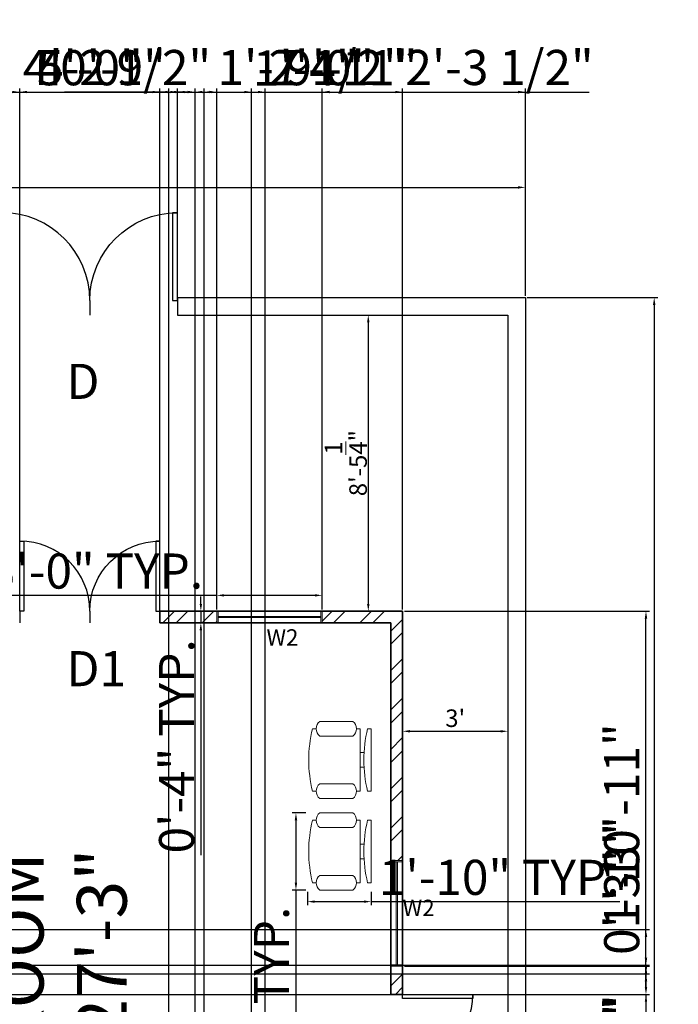
# Model space of a CAD drawing. Units: inches. Extents: x 2242 to 2870, y 1782 to 2635.
# Tile 7 of 7: x 2582 to 2807, y 2299 to 2635. Entities that reach past the tile are written whole.
import ezdxf

# ---------------------------------------------------------------- set-up
doc = ezdxf.new("R2010")
doc.units = ezdxf.units.IN
for name, color, linetype, lineweight in [('A-ANNO-DIMS', 7, 'Continuous', 18), ('A-ANNO-TEXT', 1, 'Continuous', 18), ('A-AREA-IDEN', 1, 'Continuous', 25), ('A-WALL-PATT', 253, 'Continuous', 13), ('C-PROP', 7, 'Continuous', 30), ('doors', 5, 'Continuous', 25), ('furniture', 9, 'Continuous', 18), ('walls', 7, 'Continuous', 35), ('windows', 72, 'Continuous', 18)]:
    doc.layers.add(name, color=color, linetype=linetype, lineweight=lineweight)
doc.styles.get("Standard").update_dxf_attribs({"font": 'arial.ttf'})
doc.dimstyles.new('ISO-25', dxfattribs={"dimtxt": 12, "dimasz": 2.5, "dimexe": 1.25, "dimexo": 0.625, "dimtad": 1, "dimlunit": 4, "dimtxsty": 'Standard', "dimcen": 2.5, "dimadec": 0, "dimazin": 0, "dimtfac": 1, "dimtmove": 0, "dimatfit": 3, "dimfxl": 1, "dimarcsym": 0})

# ---------------------------------------------------------------- blocks, each defined once
blk = doc.blocks.new('*U2')
for p, q in [((0, 0), (0, -5)), ((30, 0), (30, -5))]:
    blk.add_line(p, q)
blk.add_lwpolyline([(0, 0), (0, 30), (1.75, 30), (1.75, 0)], close=True)
blk.add_arc((0, 0), 30, 0, 90)
blk = doc.blocks.new('Chair - Desk')
for p, q in [((-8.5, 0), (-8.5, -1)), ((-8.5, 0), (8.5, 0)), ((8.5, 0), (8.5, -1)), ((-2, -3), (-2, -1.9355)), ((2, -1.9576), (2, -3)), ((-10.5, -5), (-10.5, -14)), ((-8.5, -3), (-8.5, -4)), ((-8.5, -3), (8.5, -3)), ((-6.5, -14), (-6.5, -5)), ((6.5, -5), (6.5, -14)), ((8.5, -3), (8.5, -4)), ((10.5, -14), (10.5, -5)), ((-8.5, -15), (-8.5, -16)), ((8.5, -15), (8.5, -16))]:
    blk.add_line(p, q)
for centre, radius, start, end in [((0, 34.625), 36.625, 256.5803, 283.4197), ((-8.5, -6.5), 2.5, 36.8699, 143.1301), ((8.5, -6.5), 2.5, 36.8699, 143.1301), ((-8.5, -12.5), 2.5, 216.8699, 323.1301), ((0, 19.625), 36.625, 256.5803, 283.4197), ((8.5, -12.5), 2.5, 216.8699, 323.1301)]:
    blk.add_arc(centre, radius, start, end)
blk = doc.blocks.new('*D15')
at = {"layer": 'A-ANNO-DIMS', "color": 0, "lineweight": -2, "transparency": 16777216}
for p, q in [((2359.16, 2540.96), (2359.16, 2579.23)), ((2755.16, 2540.96), (2755.16, 2579.23)), ((2361.66, 2577.98), (2752.66, 2577.98))]:
    blk.add_line(p, q, dxfattribs=at)
at = {"layer": 'A-ANNO-DIMS', "color": 0, "transparency": 16777216}
for points in [[(2361.66, 2578.39), (2361.66, 2577.56), (2359.16, 2577.98)], [(2752.66, 2578.39), (2752.66, 2577.56), (2755.16, 2577.98)]]:
    blk.add_solid(points, dxfattribs=at)
at = {"layer": 'Defpoints', "color": 0, "transparency": 16777216}
for p in [(2755.16, 2577.98), (2359.16, 2540.33), (2755.16, 2540.33)]:
    blk.add_point(p, dxfattribs=at)
at = {"layer": 'A-ANNO-DIMS', "color": 0, "transparency": 16777216, "insert": (2557.16, 2584.73), "char_height": 12, "attachment_point": 5}
blk.add_mtext("33'", dxfattribs=at)
blk = doc.blocks.new('*D21')
at = {"layer": 'A-ANNO-DIMS', "color": 0, "lineweight": -2, "transparency": 16777216}
for p, q in [((2693.29, 2534.33), (2702.67, 2534.33)), ((2701.42, 2531.83), (2701.42, 2435.6)), ((2693.29, 2433.1), (2702.67, 2433.1))]:
    blk.add_line(p, q, dxfattribs=at)
at = {"layer": 'A-ANNO-DIMS', "color": 0, "transparency": 16777216}
for points in [[(2701, 2531.83), (2701.83, 2531.83), (2701.42, 2534.33)], [(2701, 2435.6), (2701.83, 2435.6), (2701.42, 2433.1)]]:
    blk.add_solid(points, dxfattribs=at)
at = {"layer": 'Defpoints', "color": 0, "transparency": 16777216}
for p in [(2692.66, 2534.33), (2692.66, 2433.1), (2701.42, 2433.1)]:
    blk.add_point(p, dxfattribs=at)
at = {"layer": 'A-ANNO-DIMS', "color": 0, "transparency": 16777216, "insert": (2693.73, 2483.72), "char_height": 6, "attachment_point": 5, "rotation": 90}
blk.add_mtext('8\'-5{\\H1x;\\S1/4;}"', dxfattribs=at)
blk = doc.blocks.new('*D22')
at = {"layer": 'A-ANNO-DIMS', "color": 0, "lineweight": -2, "transparency": 16777216}
for p, q in [((2713.16, 2403.6), (2713.16, 2390.8)), ((2749.16, 2403.6), (2749.16, 2390.8)), ((2715.66, 2392.05), (2746.66, 2392.05))]:
    blk.add_line(p, q, dxfattribs=at)
at = {"layer": 'A-ANNO-DIMS', "color": 0, "transparency": 16777216}
for points in [[(2715.66, 2392.46), (2715.66, 2391.63), (2713.16, 2392.05)], [(2746.66, 2392.46), (2746.66, 2391.63), (2749.16, 2392.05)]]:
    blk.add_solid(points, dxfattribs=at)
at = {"layer": 'Defpoints', "color": 0, "transparency": 16777216}
for p in [(2713.16, 2404.22), (2749.16, 2404.22), (2749.16, 2392.05)]:
    blk.add_point(p, dxfattribs=at)
at = {"layer": 'A-ANNO-DIMS', "color": 0, "transparency": 16777216, "insert": (2731.16, 2395.74), "char_height": 6, "attachment_point": 5}
blk.add_mtext("3'", dxfattribs=at)
blk = doc.blocks.new('*D29')
at = {"layer": 'A-ANNO-DIMS', "color": 0, "lineweight": -2, "transparency": 16777216}
for p, q in [((2755.79, 2540.33), (2800.47, 2540.33)), ((2799.22, 2537.83), (2799.22, 1942.83)), ((2755.79, 1940.33), (2800.47, 1940.33))]:
    blk.add_line(p, q, dxfattribs=at)
at = {"layer": 'A-ANNO-DIMS', "color": 0, "transparency": 16777216}
for points in [[(2798.81, 2537.83), (2799.64, 2537.83), (2799.22, 2540.33)], [(2798.81, 1942.83), (2799.64, 1942.83), (2799.22, 1940.33)]]:
    blk.add_solid(points, dxfattribs=at)
at = {"layer": 'Defpoints', "color": 0, "transparency": 16777216}
for p in [(2755.16, 2540.33), (2755.16, 1940.33), (2799.22, 1940.33)]:
    blk.add_point(p, dxfattribs=at)
at = {"layer": 'A-ANNO-DIMS', "color": 0, "transparency": 16777216, "insert": (2792.47, 2240.33), "char_height": 12, "attachment_point": 5, "rotation": 90}
blk.add_mtext("50'", dxfattribs=at)
blk = doc.blocks.new('WIN-W2-36IN')
for p, q in [((0, 4), (36.12, 4)), ((0, 0), (0, 4)), ((0.5, 0), (0.5, 4)), ((35.62, 4), (35.62, 0)), ((36.12, 4), (36.12, 0)), ((36.12, 0), (0, 0)), ((0.5, 2.2), (35.62, 2.2)), ((0.5, 1.8), (35.62, 1.8))]:
    blk.add_line(p, q)
blk = doc.blocks.new('*D33')
at = {"layer": 'A-ANNO-DIMS', "color": 0, "lineweight": -2, "transparency": 16777216}
for p, q in [((2649.56, 2438.51), (2542.37, 2438.51)), ((2649.56, 2433.72), (2649.56, 2439.76)), ((2683.18, 2438.51), (2652.06, 2438.51)), ((2685.68, 2433.72), (2685.68, 2439.76))]:
    blk.add_line(p, q, dxfattribs=at)
at = {"layer": 'A-ANNO-DIMS', "color": 0, "transparency": 16777216}
for points in [[(2652.06, 2438.93), (2652.06, 2438.1), (2649.56, 2438.51)], [(2683.18, 2438.93), (2683.18, 2438.1), (2685.68, 2438.51)]]:
    blk.add_solid(points, dxfattribs=at)
at = {"layer": 'Defpoints', "color": 0, "transparency": 16777216}
for p in [(2649.56, 2438.51), (2649.56, 2433.1), (2685.68, 2433.1)]:
    blk.add_point(p, dxfattribs=at)
at = {"layer": 'A-ANNO-DIMS', "color": 0, "transparency": 16777216, "insert": (2594.72, 2445.27), "char_height": 12, "attachment_point": 5}
blk.add_mtext('W2 3\'-0" TYP.', dxfattribs=at)
blk = doc.blocks.new('*D34')
at = {"layer": 'A-ANNO-DIMS', "color": 0, "lineweight": -2, "transparency": 16777216}
for p, q in [((2644.14, 2435.6), (2644.14, 2438.1)), ((2648.94, 2433.1), (2642.89, 2433.1)), ((2644.14, 2433.1), (2644.14, 2429.1)), ((2648.94, 2429.1), (2642.89, 2429.1)), ((2644.14, 2426.6), (2644.14, 2349.7))]:
    blk.add_line(p, q, dxfattribs=at)
at = {"layer": 'A-ANNO-DIMS', "color": 0, "transparency": 16777216}
for points in [[(2643.73, 2435.6), (2644.56, 2435.6), (2644.14, 2433.1)], [(2643.73, 2426.6), (2644.56, 2426.6), (2644.14, 2429.1)]]:
    blk.add_solid(points, dxfattribs=at)
at = {"layer": 'Defpoints', "color": 0, "transparency": 16777216}
for p in [(2649.56, 2433.1), (2644.14, 2429.1), (2649.56, 2429.1)]:
    blk.add_point(p, dxfattribs=at)
at = {"layer": 'A-ANNO-DIMS', "color": 0, "transparency": 16777216, "insert": (2637.39, 2386.9), "char_height": 12, "attachment_point": 5, "rotation": 90}
blk.add_mtext('0\'-4" TYP.', dxfattribs=at)
blk = doc.blocks.new('*D45')
at = {"layer": 'A-ANNO-DIMS', "color": 0, "lineweight": -2, "transparency": 16777216}
for p, q in [((2680.01, 2364.16), (2675.42, 2364.16)), ((2676.67, 2361.66), (2676.67, 2340.27)), ((2680.01, 2337.77), (2675.42, 2337.77)), ((2676.67, 2337.77), (2676.67, 2176.23))]:
    blk.add_line(p, q, dxfattribs=at)
at = {"layer": 'A-ANNO-DIMS', "color": 0, "transparency": 16777216}
for points in [[(2676.26, 2361.66), (2677.09, 2361.66), (2676.67, 2364.16)], [(2676.26, 2340.27), (2677.09, 2340.27), (2676.67, 2337.77)]]:
    blk.add_solid(points, dxfattribs=at)
at = {"layer": 'Defpoints', "color": 0, "transparency": 16777216}
for p in [(2680.63, 2364.16), (2676.67, 2337.77), (2680.63, 2337.77)]:
    blk.add_point(p, dxfattribs=at)
at = {"layer": 'A-ANNO-DIMS', "color": 0, "transparency": 16777216, "insert": (2669.84, 2255.75), "char_height": 12, "attachment_point": 5, "rotation": 90}
blk.add_mtext('CHAIR 2\'-2 1/2" TYP.', dxfattribs=at)
blk = doc.blocks.new('*D46')
at = {"layer": 'A-ANNO-DIMS', "color": 0, "lineweight": -2, "transparency": 16777216}
for p, q in [((2680.63, 2337.14), (2680.63, 2332.56)), ((2702.42, 2337.14), (2702.42, 2332.56)), ((2683.13, 2333.81), (2699.92, 2333.81)), ((2702.42, 2333.81), (2787.51, 2333.81))]:
    blk.add_line(p, q, dxfattribs=at)
at = {"layer": 'A-ANNO-DIMS', "color": 0, "transparency": 16777216}
for points in [[(2683.13, 2334.22), (2683.13, 2333.39), (2680.63, 2333.81)], [(2699.92, 2334.22), (2699.92, 2333.39), (2702.42, 2333.81)]]:
    blk.add_solid(points, dxfattribs=at)
at = {"layer": 'Defpoints', "color": 0, "transparency": 16777216}
for p in [(2680.63, 2337.77), (2702.42, 2337.77), (2702.42, 2333.81)]:
    blk.add_point(p, dxfattribs=at)
at = {"layer": 'A-ANNO-DIMS', "color": 0, "transparency": 16777216, "insert": (2746.21, 2340.56), "char_height": 12, "attachment_point": 5}
blk.add_mtext('1\'-10" TYP.', dxfattribs=at)
blk = doc.blocks.new('*D59')
at = {"layer": 'A-ANNO-DIMS', "color": 0, "lineweight": -2, "transparency": 16777216}
for p, q in [((2576.16, 2540.96), (2576.16, 2611.83)), ((2578.66, 2610.58), (2633.66, 2610.58)), ((2636.16, 2540.96), (2636.16, 2611.83))]:
    blk.add_line(p, q, dxfattribs=at)
at = {"layer": 'A-ANNO-DIMS', "color": 0, "transparency": 16777216}
for points in [[(2578.66, 2611), (2578.66, 2610.17), (2576.16, 2610.58)], [(2633.66, 2611), (2633.66, 2610.17), (2636.16, 2610.58)]]:
    blk.add_solid(points, dxfattribs=at)
at = {"layer": 'Defpoints', "color": 0, "transparency": 16777216}
for p in [(2636.16, 2610.58), (2576.16, 2540.33), (2636.16, 2540.33)]:
    blk.add_point(p, dxfattribs=at)
at = {"layer": 'A-ANNO-DIMS', "color": 0, "transparency": 16777216, "insert": (2606.16, 2617.34), "char_height": 12, "attachment_point": 5}
blk.add_mtext('5\'-0"', dxfattribs=at)
blk = doc.blocks.new('*D60')
at = {"layer": 'A-ANNO-DIMS', "color": 0, "lineweight": -2, "transparency": 16777216}
for p, q in [((2636.16, 2540.96), (2636.16, 2611.83)), ((2638.66, 2610.58), (2752.66, 2610.58)), ((2755.16, 2540.96), (2755.16, 2611.83))]:
    blk.add_line(p, q, dxfattribs=at)
at = {"layer": 'A-ANNO-DIMS', "color": 0, "transparency": 16777216}
for points in [[(2638.66, 2611), (2638.66, 2610.17), (2636.16, 2610.58)], [(2752.66, 2611), (2752.66, 2610.17), (2755.16, 2610.58)]]:
    blk.add_solid(points, dxfattribs=at)
at = {"layer": 'Defpoints', "color": 0, "transparency": 16777216}
for p in [(2755.16, 2610.58), (2636.16, 2540.33), (2755.16, 2540.33)]:
    blk.add_point(p, dxfattribs=at)
at = {"layer": 'A-ANNO-DIMS', "color": 0, "transparency": 16777216, "insert": (2695.66, 2617.34), "char_height": 12, "attachment_point": 5}
blk.add_mtext('9\'-11"', dxfattribs=at)
blk = doc.blocks.new('*D61')
at = {"layer": 'A-ANNO-DIMS', "color": 0, "lineweight": -2, "transparency": 16777216}
for p, q in [((2582.16, 2433.72), (2582.16, 2611.83)), ((2584.66, 2610.58), (2627.66, 2610.58)), ((2630.16, 2433.72), (2630.16, 2611.83))]:
    blk.add_line(p, q, dxfattribs=at)
at = {"layer": 'A-ANNO-DIMS', "color": 0, "transparency": 16777216}
for points in [[(2584.66, 2611), (2584.66, 2610.17), (2582.16, 2610.58)], [(2627.66, 2611), (2627.66, 2610.17), (2630.16, 2610.58)]]:
    blk.add_solid(points, dxfattribs=at)
at = {"layer": 'Defpoints', "color": 0, "transparency": 16777216}
for p in [(2630.16, 2610.58), (2582.16, 2433.1), (2630.16, 2433.1)]:
    blk.add_point(p, dxfattribs=at)
at = {"layer": 'A-ANNO-DIMS', "color": 0, "transparency": 16777216, "insert": (2606.16, 2617.34), "char_height": 12, "attachment_point": 5}
blk.add_mtext('4\'-0"', dxfattribs=at)
blk = doc.blocks.new('*D62')
at = {"layer": 'A-ANNO-DIMS', "color": 0, "lineweight": -2, "transparency": 16777216}
for p, q in [((2537.37, 2302.1), (2797.66, 2302.1)), ((2796.41, 2299.6), (2796.41, 2268.6)), ((2537.37, 2266.1), (2797.66, 2266.1))]:
    blk.add_line(p, q, dxfattribs=at)
at = {"layer": 'A-ANNO-DIMS', "color": 0, "transparency": 16777216}
for points in [[(2796, 2299.6), (2796.83, 2299.6), (2796.41, 2302.1)], [(2796, 2268.6), (2796.83, 2268.6), (2796.41, 2266.1)]]:
    blk.add_solid(points, dxfattribs=at)
at = {"layer": 'Defpoints', "color": 0, "transparency": 16777216}
for p in [(2536.74, 2302.1), (2536.74, 2266.1), (2796.41, 2266.1)]:
    blk.add_point(p, dxfattribs=at)
at = {"layer": 'A-ANNO-DIMS', "color": 0, "transparency": 16777216, "insert": (2789.66, 2284.1), "char_height": 12, "attachment_point": 5, "rotation": 90}
blk.add_mtext('3\'-0"', dxfattribs=at)
blk = doc.blocks.new('*D64')
at = {"layer": 'A-ANNO-DIMS', "color": 0, "lineweight": -2, "transparency": 16777216}
for p, q in [((2642.16, 2049.72), (2642.16, 2611.83)), ((2644.66, 2610.58), (2663.66, 2610.58)), ((2666.16, 2049.72), (2666.16, 2611.83)), ((2666.16, 2610.58), (2702.02, 2610.58))]:
    blk.add_line(p, q, dxfattribs=at)
at = {"layer": 'A-ANNO-DIMS', "color": 0, "transparency": 16777216}
for points in [[(2644.66, 2611), (2644.66, 2610.17), (2642.16, 2610.58)], [(2663.66, 2611), (2663.66, 2610.17), (2666.16, 2610.58)]]:
    blk.add_solid(points, dxfattribs=at)
at = {"layer": 'Defpoints', "color": 0, "transparency": 16777216}
for p in [(2666.16, 2610.58), (2642.16, 2049.1), (2666.16, 2049.1)]:
    blk.add_point(p, dxfattribs=at)
at = {"layer": 'A-ANNO-DIMS', "color": 0, "transparency": 16777216, "insert": (2685.34, 2617.34), "char_height": 12, "attachment_point": 5}
blk.add_mtext('2\'-0"', dxfattribs=at)
blk = doc.blocks.new('*D65')
at = {"layer": 'A-ANNO-DIMS', "color": 0, "lineweight": -2, "transparency": 16777216}
for p, q in [((2713.79, 2433.1), (2797.66, 2433.1)), ((2796.41, 2304.6), (2796.41, 2430.6)), ((2713.79, 2302.1), (2797.66, 2302.1))]:
    blk.add_line(p, q, dxfattribs=at)
at = {"layer": 'A-ANNO-DIMS', "color": 0, "transparency": 16777216}
for points in [[(2796, 2430.6), (2796.83, 2430.6), (2796.41, 2433.1)], [(2796, 2304.6), (2796.83, 2304.6), (2796.41, 2302.1)]]:
    blk.add_solid(points, dxfattribs=at)
at = {"layer": 'Defpoints', "color": 0, "transparency": 16777216}
for p in [(2713.16, 2433.1), (2796.41, 2433.1), (2713.16, 2302.1)]:
    blk.add_point(p, dxfattribs=at)
at = {"layer": 'A-ANNO-DIMS', "color": 0, "transparency": 16777216, "insert": (2789.66, 2367.6), "char_height": 12, "attachment_point": 5, "rotation": 90}
blk.add_mtext('10\'-11"', dxfattribs=at)
blk = doc.blocks.new('*D66')
at = {"layer": 'A-ANNO-DIMS', "color": 0, "lineweight": -2, "transparency": 16777216}
for p, q in [((2713.79, 2311.76), (2797.66, 2311.76)), ((2796.41, 2309.26), (2796.41, 2304.6)), ((2713.79, 2302.1), (2797.66, 2302.1)), ((2796.41, 2302.1), (2796.41, 2238.49))]:
    blk.add_line(p, q, dxfattribs=at)
at = {"layer": 'A-ANNO-DIMS', "color": 0, "transparency": 16777216}
for points in [[(2796, 2309.26), (2796.83, 2309.26), (2796.41, 2311.76)], [(2796, 2304.6), (2796.83, 2304.6), (2796.41, 2302.1)]]:
    blk.add_solid(points, dxfattribs=at)
at = {"layer": 'Defpoints', "color": 0, "transparency": 16777216}
for p in [(2713.16, 2311.76), (2713.16, 2302.1), (2796.41, 2302.1)]:
    blk.add_point(p, dxfattribs=at)
at = {"layer": 'A-ANNO-DIMS', "color": 0, "transparency": 16777216, "insert": (2789.58, 2269.04), "char_height": 12, "attachment_point": 5, "rotation": 90}
blk.add_mtext('0\'-9 1/2"', dxfattribs=at)
blk = doc.blocks.new('*D69')
at = {"layer": 'A-ANNO-DIMS', "color": 0, "lineweight": -2, "transparency": 16777216}
for p, q in [((2630.16, 2433.72), (2630.16, 2611.83)), ((2632.66, 2610.58), (2647.06, 2610.58)), ((2649.56, 2433.72), (2649.56, 2611.83)), ((2649.56, 2610.58), (2712.04, 2610.58))]:
    blk.add_line(p, q, dxfattribs=at)
at = {"layer": 'A-ANNO-DIMS', "color": 0, "transparency": 16777216}
for points in [[(2632.66, 2611), (2632.66, 2610.17), (2630.16, 2610.58)], [(2647.06, 2611), (2647.06, 2610.17), (2649.56, 2610.58)]]:
    blk.add_solid(points, dxfattribs=at)
at = {"layer": 'Defpoints', "color": 0, "transparency": 16777216}
for p in [(2649.56, 2610.58), (2630.16, 2433.1), (2649.56, 2433.1)]:
    blk.add_point(p, dxfattribs=at)
at = {"layer": 'A-ANNO-DIMS', "color": 0, "transparency": 16777216, "insert": (2682.05, 2617.41), "char_height": 12, "attachment_point": 5}
blk.add_mtext('1\'-7 1/2"', dxfattribs=at)
blk = doc.blocks.new('*D70')
at = {"layer": 'A-ANNO-DIMS', "color": 0, "lineweight": -2, "transparency": 16777216}
for p, q in [((2685.68, 2433.72), (2685.68, 2611.83)), ((2688.18, 2610.58), (2710.66, 2610.58)), ((2713.16, 2433.72), (2713.16, 2611.83)), ((2713.16, 2610.58), (2776.98, 2610.58))]:
    blk.add_line(p, q, dxfattribs=at)
at = {"layer": 'A-ANNO-DIMS', "color": 0, "transparency": 16777216}
for points in [[(2688.18, 2611), (2688.18, 2610.17), (2685.68, 2610.58)], [(2710.66, 2611), (2710.66, 2610.17), (2713.16, 2610.58)]]:
    blk.add_solid(points, dxfattribs=at)
at = {"layer": 'Defpoints', "color": 0, "transparency": 16777216}
for p in [(2713.16, 2610.58), (2685.68, 2433.1), (2713.16, 2433.1)]:
    blk.add_point(p, dxfattribs=at)
at = {"layer": 'A-ANNO-DIMS', "color": 0, "transparency": 16777216, "insert": (2746.32, 2617.42), "char_height": 12, "attachment_point": 5}
blk.add_mtext('2\'-3 1/2"', dxfattribs=at)
blk = doc.blocks.new('*D71')
at = {"layer": 'A-ANNO-DIMS', "color": 0, "lineweight": -2, "transparency": 16777216}
for p, q in [((2531.58, 2433.72), (2531.58, 2611.83)), ((2534.08, 2610.58), (2579.66, 2610.58)), ((2582.16, 2433.72), (2582.16, 2611.83)), ((2582.16, 2610.58), (2646.26, 2610.58))]:
    blk.add_line(p, q, dxfattribs=at)
at = {"layer": 'A-ANNO-DIMS', "color": 0, "transparency": 16777216}
for points in [[(2534.08, 2611), (2534.08, 2610.17), (2531.58, 2610.58)], [(2579.66, 2611), (2579.66, 2610.17), (2582.16, 2610.58)]]:
    blk.add_solid(points, dxfattribs=at)
at = {"layer": 'Defpoints', "color": 0, "transparency": 16777216}
for p in [(2582.16, 2610.58), (2531.58, 2433.1), (2582.16, 2433.1)]:
    blk.add_point(p, dxfattribs=at)
at = {"layer": 'A-ANNO-DIMS', "color": 0, "transparency": 16777216, "insert": (2615.46, 2617.41), "char_height": 12, "attachment_point": 5}
blk.add_mtext('4\'-2 1/2"', dxfattribs=at)
blk = doc.blocks.new('*D74')
at = {"layer": 'A-ANNO-DIMS', "color": 0, "lineweight": -2, "transparency": 16777216}
for p, q in [((2645.26, 2208.5), (2645.26, 2611.83)), ((2647.76, 2610.58), (2658.99, 2610.58)), ((2661.49, 2208.5), (2661.49, 2611.83)), ((2661.49, 2610.58), (2696.01, 2610.58))]:
    blk.add_line(p, q, dxfattribs=at)
at = {"layer": 'A-ANNO-DIMS', "color": 0, "transparency": 16777216}
for points in [[(2647.76, 2611), (2647.76, 2610.17), (2645.26, 2610.58)], [(2658.99, 2611), (2658.99, 2610.17), (2661.49, 2610.58)]]:
    blk.add_solid(points, dxfattribs=at)
at = {"layer": 'Defpoints', "color": 0, "transparency": 16777216}
for p in [(2661.49, 2610.58), (2645.26, 2207.87), (2661.49, 2207.87)]:
    blk.add_point(p, dxfattribs=at)
at = {"layer": 'A-ANNO-DIMS', "color": 0, "transparency": 16777216, "insert": (2680, 2617.23), "char_height": 12, "attachment_point": 5}
blk.add_mtext('1\'-4"', dxfattribs=at)
blk = doc.blocks.new('*D79')
at = {"layer": 'A-ANNO-DIMS', "color": 0, "lineweight": -2, "transparency": 16777216}
for p, q in [((2796.41, 2324.23), (2796.41, 2358.75)), ((2393.37, 2324.23), (2797.66, 2324.23)), ((2796.41, 2311.6), (2796.41, 2321.73)), ((2393.37, 2309.1), (2797.66, 2309.1))]:
    blk.add_line(p, q, dxfattribs=at)
at = {"layer": 'A-ANNO-DIMS', "color": 0, "transparency": 16777216}
for points in [[(2796, 2321.73), (2796.83, 2321.73), (2796.41, 2324.23)], [(2796, 2311.6), (2796.83, 2311.6), (2796.41, 2309.1)]]:
    blk.add_solid(points, dxfattribs=at)
at = {"layer": 'Defpoints', "color": 0, "transparency": 16777216}
for p in [(2392.74, 2324.23), (2796.41, 2324.23), (2392.74, 2309.1)]:
    blk.add_point(p, dxfattribs=at)
at = {"layer": 'A-ANNO-DIMS', "color": 0, "transparency": 16777216, "insert": (2789.66, 2342.74), "char_height": 12, "attachment_point": 5, "rotation": 90}
blk.add_mtext('1\'-3"', dxfattribs=at)
blk = doc.blocks.new('*D82')
at = {"layer": 'A-ANNO-DIMS', "color": 0, "lineweight": -2, "transparency": 16777216}
for p, q in [((2633.16, 2610.58), (2597.51, 2610.58)), ((2633.16, 2049.72), (2633.16, 2611.83)), ((2639.66, 2610.58), (2635.66, 2610.58)), ((2642.16, 2049.72), (2642.16, 2611.83))]:
    blk.add_line(p, q, dxfattribs=at)
at = {"layer": 'A-ANNO-DIMS', "color": 0, "transparency": 16777216}
for points in [[(2635.66, 2611), (2635.66, 2610.17), (2633.16, 2610.58)], [(2639.66, 2611), (2639.66, 2610.17), (2642.16, 2610.58)]]:
    blk.add_solid(points, dxfattribs=at)
at = {"layer": 'Defpoints', "color": 0, "transparency": 16777216}
for p in [(2633.16, 2610.58), (2633.16, 2049.1), (2642.16, 2049.1)]:
    blk.add_point(p, dxfattribs=at)
at = {"layer": 'A-ANNO-DIMS', "color": 0, "transparency": 16777216, "insert": (2614.09, 2617.34), "char_height": 12, "attachment_point": 5}
blk.add_mtext('0\'-9"', dxfattribs=at)
blk = doc.blocks.new('*D83')
at = {"layer": 'A-ANNO-DIMS', "color": 0, "lineweight": -2, "transparency": 16777216}
for p, q in [((2796.41, 2314.6), (2796.41, 2350.25)), ((2537.37, 2312.1), (2797.66, 2312.1)), ((2796.41, 2309.1), (2796.41, 2312.1)), ((2537.37, 2309.1), (2797.66, 2309.1)), ((2796.41, 2306.6), (2796.41, 2304.1))]:
    blk.add_line(p, q, dxfattribs=at)
at = {"layer": 'A-ANNO-DIMS', "color": 0, "transparency": 16777216}
for points in [[(2796, 2314.6), (2796.83, 2314.6), (2796.41, 2312.1)], [(2796, 2306.6), (2796.83, 2306.6), (2796.41, 2309.1)]]:
    blk.add_solid(points, dxfattribs=at)
at = {"layer": 'Defpoints', "color": 0, "transparency": 16777216}
for p in [(2536.74, 2312.1), (2796.41, 2312.1), (2536.74, 2309.1)]:
    blk.add_point(p, dxfattribs=at)
at = {"layer": 'A-ANNO-DIMS', "color": 0, "transparency": 16777216, "insert": (2789.66, 2333.67), "char_height": 12, "attachment_point": 5, "rotation": 90}
blk.add_mtext('0\'-3"', dxfattribs=at)

msp = doc.modelspace()

# ---------------------------------------------------------------- hatches: boundary and pattern name
at = {"layer": 'A-WALL-PATT'}
h = msp.add_hatch(dxfattribs=at)
h.set_pattern_fill('ANSI32', color=256)
h.paths.add_polyline_path([(2649.562, 2433.097), (2630.164, 2433.097), (2630.164, 2429.097), (2649.562, 2429.097)])
h = msp.add_hatch(dxfattribs=at)
h.set_pattern_fill('ANSI32', color=256)
h.paths.add_polyline_path([(2713.164, 2433.097), (2685.678, 2433.097), (2685.678, 2429.097), (2709.164, 2429.097), (2709.164, 2347.877), (2713.164, 2347.877)])
h = msp.add_hatch(dxfattribs=at)
h.set_pattern_fill('ANSI32', color=256)
h.paths.add_polyline_path([(2713.164, 2311.761), (2709.164, 2311.761), (2709.164, 2302.097), (2713.164, 2302.097)])

# ---------------------------------------------------------------- linework, layer by layer
at = {"layer": 'C-PROP'}
for p, q in [((2636.164, 2540.335), (2636.164, 2534.335)), ((2636.164, 2540.335), (2755.164, 2540.335)), ((2755.164, 2540.335), (2755.164, 1940.335)), ((2636.164, 2534.335), (2749.164, 2534.335)), ((2749.164, 2534.335), (2749.164, 1945.097))]:
    msp.add_line(p, q, dxfattribs=at)
at = {"layer": 'walls'}
for p, q in [((2713.164, 2433.097), (2630.164, 2433.097)), ((2630.164, 2433.097), (2630.164, 2429.097)), ((2713.164, 2433.097), (2713.164, 2302.097)), ((2709.164, 2429.097), (2630.164, 2429.097)), ((2630.164, 2429.097), (2630.164, 2429.097)), ((2709.164, 2429.097), (2709.164, 2302.097)), ((2709.164, 2302.097), (2713.164, 2302.097))]:
    msp.add_line(p, q, dxfattribs=at)

# ---------------------------------------------------------------- block references
at = {"layer": 'doors'}
msp.add_blockref('*U2', (2576.164, 2539.335), dxfattribs=at)
at = {"layer": 'doors', "xscale": -1}
msp.add_blockref('*U2', (2636.164, 2539.335), dxfattribs=at)
at = {"layer": 'doors', "yscale": 0.8, "zscale": 0.8}
for p, xscale in [((2582.164, 2433.097), 0.8), ((2630.164, 2433.097), -0.8)]:
    msp.add_blockref('*U2', p, dxfattribs=dict(at, xscale=xscale))
at = {"layer": 'doors', "xscale": 0.8, "yscale": 0.8, "zscale": 0.8, "rotation": 270}
msp.add_blockref('*U2', (2713.164, 2302.097), dxfattribs=at)
at = {"layer": 'furniture', "xscale": 1.256752467488209, "yscale": 1.256752467488209, "zscale": 1.256752467488209, "rotation": 270}
for p in [(2702.417, 2382.247), (2702.417, 2350.963)]:
    msp.add_blockref('Chair - Desk', p, dxfattribs=at)
at = {"layer": 'windows'}
for p, rotation in [((2685.678, 2433.098), 180), ((2713.164, 2311.76), 89.99999999999889)]:
    msp.add_blockref('WIN-W2-36IN', p, dxfattribs=dict(at, rotation=rotation))

# ---------------------------------------------------------------- texts
at = {"layer": 'A-ANNO-TEXT', "attachment_point": 1}
for s, width, gutter_width, insert, char_height in [('D', 2.16795, 12.5, (2598.203, 2517.661), 12), ('W2', 0.54422, 27.96, (2666.59, 2426.924), 5.5921), ('D1', 2.16795, 12.5, (2598.203, 2419.45), 12), ('W2', 0.54422, 27.96, (2713.164, 2334.465), 5.5921)]:
    msp.add_mtext_dynamic_manual_height_columns(s, width=width, gutter_width=gutter_width, heights=[0], dxfattribs=dict(at, insert=insert, char_height=char_height))
at = {"layer": 'A-AREA-IDEN', "insert": (2573.308, 2210.091), "char_height": 17.04609, "attachment_point": 1, "rotation": 90}
msp.add_mtext_dynamic_manual_height_columns('LIVINGROOM\\P14\'-3"X27\'-3"', width=6.2214, gutter_width=17.756, heights=[0], dxfattribs=at)

# ---------------------------------------------------------------- dimensions: what is measured, and where the dimension line sits
at = {"layer": 'A-ANNO-DIMS'}
for base, p1, p2, override, picture, middle in [((2582.164, 2610.585), (2531.584, 2433.097), (2582.164, 2433.097), {"dimdec": 1, "dimlfac": 1, "dimrnd": 0, "dimzin": 1, "dimdsep": 46, "dimlunit": 4, "dimfrac": 2}, '*D71', (2615.46, 2617.414)), ((2649.562, 2610.585), (2630.164, 2433.097), (2649.562, 2433.097), {"dimdec": 1, "dimlfac": 1, "dimrnd": 0, "dimzin": 1, "dimdsep": 46, "dimlunit": 4, "dimfrac": 2}, '*D69', (2682.052, 2617.414)), ((2713.164, 2610.585), (2685.678, 2433.097), (2713.164, 2433.097), {"dimdec": 1, "dimlfac": 1, "dimrnd": 0, "dimzin": 1, "dimdsep": 46, "dimlunit": 4, "dimfrac": 2}, '*D70', (2746.321, 2617.418)), ((2636.164, 2610.585), (2576.164, 2540.335), (2636.164, 2540.335), {"dimdec": 1, "dimlfac": 1, "dimrnd": 0, "dimzin": 1, "dimdsep": 46, "dimlunit": 4, "dimfrac": 2}, '*D59', (2606.164, 2617.337)), ((2630.164, 2610.585), (2582.164, 2433.097), (2630.164, 2433.097), {"dimdec": 1, "dimlfac": 1, "dimrnd": 0, "dimzin": 1, "dimdsep": 46, "dimlunit": 4, "dimfrac": 2}, '*D61', (2606.164, 2617.337)), ((2633.164, 2610.585), (2642.164, 2049.097), (2633.164, 2049.097), {"dimdec": 1, "dimlfac": 1, "dimrnd": 0, "dimzin": 1, "dimdsep": 46, "dimlunit": 4, "dimfrac": 2}, '*D82', (2614.089, 2617.337)), ((2755.164, 2610.585), (2636.164, 2540.335), (2755.164, 2540.335), {"dimdec": 1, "dimlfac": 1, "dimrnd": 0, "dimzin": 1, "dimdsep": 46, "dimlunit": 4, "dimfrac": 2}, '*D60', (2695.664, 2617.337)), ((2666.164, 2610.585), (2642.164, 2049.097), (2666.164, 2049.097), {"dimdec": 1, "dimlfac": 1, "dimrnd": 0, "dimzin": 1, "dimdsep": 46, "dimlunit": 4, "dimfrac": 2}, '*D64', (2685.34, 2617.337)), ((2661.491, 2610.585), (2645.258, 2207.871), (2661.491, 2207.871), {"dimdec": 1, "dimlfac": 1, "dimrnd": 0, "dimzin": 1, "dimdsep": 46, "dimlunit": 4, "dimfrac": 2}, '*D74', (2680, 2617.234)), ((2755.164, 2577.978), (2359.164, 2540.335), (2755.164, 2540.335), {"dimclrd": 0, "dimclre": 0, "dimclrt": 0}, '*D15', (2557.164, 2584.734)), ((2749.164, 2392.046), (2713.164, 2404.225), (2749.164, 2404.225), {"dimtxt": 6, "dimclrd": 0, "dimclre": 0, "dimclrt": 0}, '*D22', (2731.164, 2395.737))]:
    dim = msp.add_linear_dim(base=base, p1=p1, p2=p2, dimstyle='ISO-25', override=override, dxfattribs=at)
    dim.commit()
    dim.dimension.update_dxf_attribs({"geometry": picture, "text_midpoint": middle})
for base, p1, p2, override, picture, middle in [((2799.223, 1940.335), (2755.164, 2540.335), (2755.164, 1940.335), {"dimclrd": 0, "dimclre": 0, "dimclrt": 0}, '*D29', (2792.471, 2240.335)), ((2701.418, 2433.097), (2692.664, 2534.335), (2692.664, 2433.097), {"dimtxt": 6, "dimclrd": 0, "dimclre": 0, "dimclrt": 0}, '*D21', (2693.73, 2483.716)), ((2796.414, 2433.097), (2713.164, 2302.097), (2713.164, 2433.097), {"dimdec": 1, "dimlfac": 1, "dimrnd": 0, "dimzin": 1, "dimdsep": 46, "dimlunit": 4, "dimfrac": 2}, '*D65', (2789.662, 2367.597)), ((2796.414, 2324.226), (2392.745, 2309.097), (2392.745, 2324.226), {"dimdec": 1, "dimlfac": 1, "dimrnd": 0, "dimzin": 1, "dimdsep": 46, "dimlunit": 4, "dimfrac": 2}, '*D79', (2789.658, 2342.736)), ((2796.414, 2312.097), (2536.745, 2309.097), (2536.745, 2312.097), {"dimdec": 1, "dimlfac": 1, "dimrnd": 0, "dimzin": 1, "dimdsep": 46, "dimlunit": 4, "dimfrac": 2}, '*D83', (2789.658, 2333.672)), ((2796.414, 2302.097), (2713.164, 2311.761), (2713.164, 2302.097), {"dimdec": 1, "dimlfac": 1, "dimrnd": 0, "dimzin": 1, "dimdsep": 46, "dimlunit": 4, "dimfrac": 2}, '*D66', (2789.584, 2269.042)), ((2796.414, 2266.097), (2536.745, 2302.097), (2536.745, 2266.097), {"dimdec": 1, "dimlfac": 1, "dimrnd": 0, "dimzin": 1, "dimdsep": 46, "dimlunit": 4, "dimfrac": 2}, '*D62', (2789.658, 2284.097))]:
    dim = msp.add_linear_dim(base=base, p1=p1, p2=p2, angle=90, dimstyle='ISO-25', override=override, dxfattribs=at)
    dim.commit()
    dim.dimension.update_dxf_attribs({"geometry": picture, "text_midpoint": middle})
for base, p1, p2, angle, text, picture, middle in [((2649.562, 2438.515), (2685.678, 2433.097), (2649.562, 2433.097), 180, 'W2 <> TYP.', '*D33', (2594.716, 2445.271)), ((2644.144, 2429.097), (2649.562, 2433.097), (2649.562, 2429.097), 270, '<> TYP.', '*D34', (2637.393, 2386.899)), ((2676.674, 2337.767), (2680.633, 2364.159), (2680.633, 2337.767), 270, 'CHAIR <> TYP.', '*D45', (2669.845, 2255.75))]:
    dim = msp.add_linear_dim(base=base, p1=p1, p2=p2, angle=angle, text=text, dimstyle='ISO-25', override={"dimdec": 1, "dimlfac": 1, "dimrnd": 0, "dimzin": 1, "dimdsep": 46, "dimlunit": 4, "dimfrac": 2}, dxfattribs=at)
    dim.commit()
    dim.dimension.update_dxf_attribs({"geometry": picture, "text_midpoint": middle})
dim = msp.add_linear_dim(base=(2702.417, 2333.808), p1=(2680.633, 2337.767), p2=(2702.417, 2337.767), text='<> TYP.', dimstyle='ISO-25', override={"dimdec": 1, "dimlfac": 1, "dimrnd": 0, "dimzin": 1, "dimdsep": 46, "dimlunit": 4, "dimfrac": 2}, dxfattribs=at)
dim.commit()
dim.dimension.update_dxf_attribs({"geometry": '*D46', "text_midpoint": (2746.212, 2340.56)})

doc.saveas('drawing.dxf')
